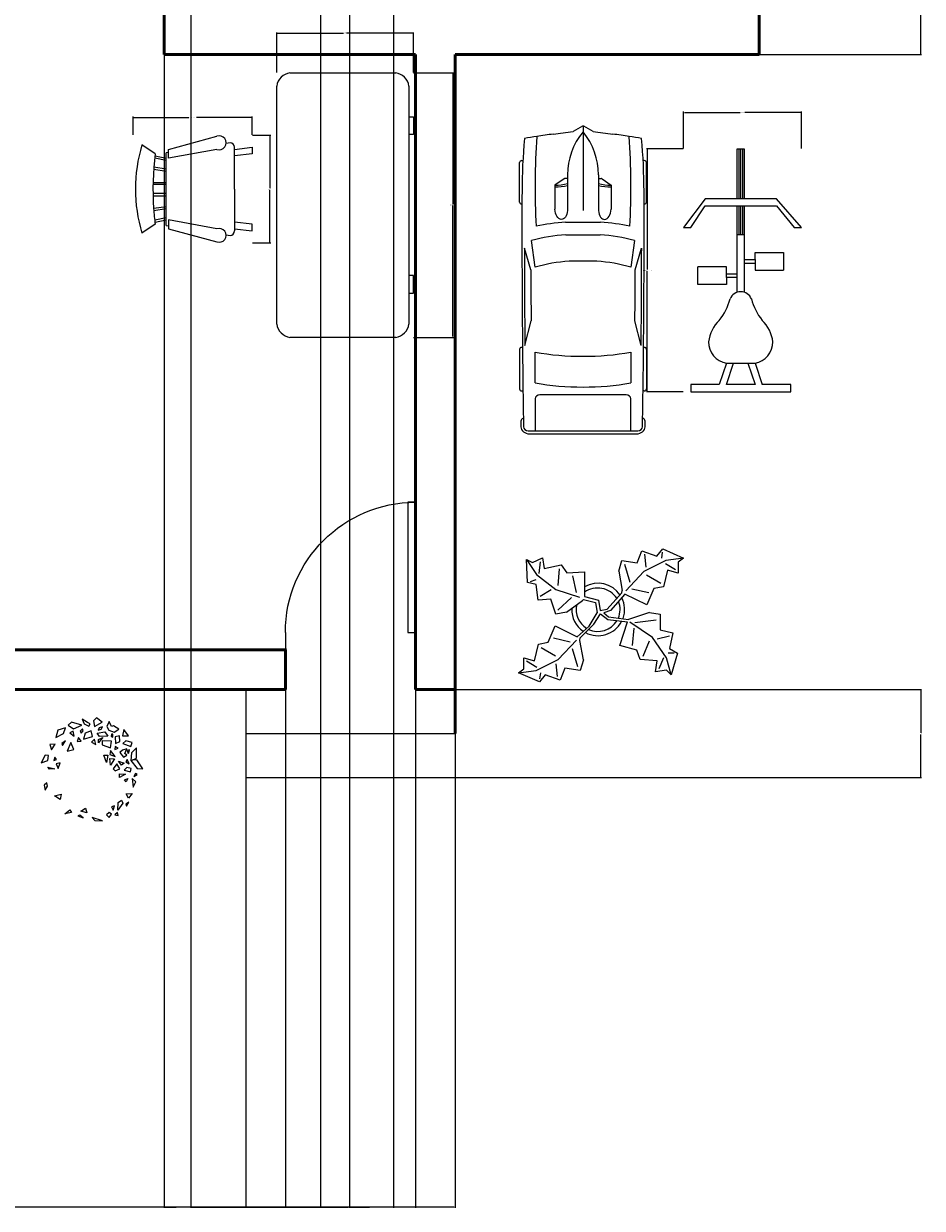
# Model space of a CAD drawing. Units: inches. Extents: x 177 to 602, y 30 to 608.
# Tile 2 of 4: x 398 to 602, y 30 to 299. Entities that reach past the tile are written whole.
import ezdxf

# ---------------------------------------------------------------- set-up
doc = ezdxf.new("R2010")
doc.units = ezdxf.units.IN
doc.header["$MEASUREMENT"] = 0
for name, color, linetype, lineweight in [('A-ANNO-DIMS', 2, 'Continuous', 18), ('A-DOOR', 3, 'Continuous', 25), ('A-EQPM', 9, 'Continuous', 18), ('A-FLOR-STRS', 7, 'Continuous', 25), ('A-FURN', 8, 'Continuous', 18), ('A-WALL', 7, 'Continuous', 50), ('C-PRKG-VEHL', 8, 'Continuous', 13), ('L-PLNT', 94, 'Continuous', 13)]:
    doc.layers.add(name, color=color, linetype=linetype, lineweight=lineweight)
doc.styles.get("Standard").update_dxf_attribs({"font": 'arial.ttf'})
doc.dimstyles.get("Standard").update_dxf_attribs({"dimtxt": 0.18, "dimasz": 0.18, "dimexe": 0.18, "dimexo": 0.0625, "dimgap": 0.09, "dimtad": 0, "dimtih": 1, "dimtoh": 1, "dimdec": 1, "dimzin": 0, "dimdsep": 46, "dimlunit": 4, "dimtxsty": 'Standard', "dimcen": 0.09, "dimadec": 0, "dimazin": 0, "dimtfac": 1, "dimtdec": 1, "dimtofl": 0, "dimtmove": 0, "dimatfit": 3, "dimfxl": 1, "dimtolj": 1, "dimtzin": 0, "dimarcsym": 0})

# ---------------------------------------------------------------- blocks, each defined once
blk = doc.blocks.new('*U3')
for p, q in [((-750, 0), (-750, 100)), ((0, 0), (0, 100))]:
    blk.add_line(p, q)
blk.add_lwpolyline([(0, 0), (0, -750), (-43.75, -750), (-43.75, 0)], close=True)
blk.add_arc((0, 0), 750, 180, 270)
blk = doc.blocks.new('*U9')
for points in [[(-4.43, 11.05), (-5.18, 10.36), (-3.96, 9.49), (-2.07, 10.36)], [(-2, 11.66), (-1.6, 10.62), (-0.52, 10.1), (-0.18, 10.62), (-0.79, 10.96)], [(1.24, 12), (0.56, 11.31), (0.76, 10.01), (2.52, 11.05)], [(4.14, 11.14), (3.6, 10.01), (4, 9.23), (5.22, 8.71), (6.3, 9.41), (5.08, 10.19), (4.61, 10.01)], [(-5.78, 9.75), (-7.54, 9.23), (-8.01, 7.5), (-6.26, 8.45)], [(-4.84, 8.63), (-3.83, 7.85), (-4.03, 8.97)], [(-1.94, 9.49), (-2.48, 8.97), (-2.27, 8.54), (-1.8, 9.06)], [(0.02, 9.06), (-1.33, 8.54), (-1.73, 7.16), (0.29, 7.76)], [(1.37, 8.54), (3.13, 8.8), (3.8, 7.85), (1.91, 7.76)], [(2.59, 9.93), (1.84, 9.75), (1.64, 9.23), (2.32, 9.41)], [(4.61, 8.28), (4.54, 7.76), (4.95, 7.59), (4.95, 8.28)], [(7.45, 9.32), (7.11, 7.94), (8.52, 7.94)], [(-8.14, 6.03), (-9.36, 5.95), (-9.02, 4.73)], [(-5.78, 6.81), (-6.66, 6.21), (-6.52, 5.69)], [(-4.57, 6.38), (-5.45, 4.47), (-3.89, 4.82)], [(-2.88, 7.5), (-3.15, 6.64), (-2.27, 6.72)], [(0.76, 7.16), (0.09, 6.46), (1.1, 5.95)], [(1.71, 6.29), (1.71, 7.07), (2.65, 7.5), (2.11, 6.9)], [(2.52, 6.81), (2.52, 5.86), (4.41, 5.17), (4.61, 6.72)], [(5.49, 5.51), (5.42, 4.82), (6.16, 5.08)], [(6.43, 7.94), (5.49, 7.68), (5.56, 6.21), (6.5, 6.64)], [(7.85, 6.81), (7.18, 6.21), (9, 5.51), (9.33, 6.38)], [(-11.32, 1.79), (-9.83, 2.31), (-9.63, 3.44), (-10.44, 3.52)], [(-8.21, 3.09), (-8.48, 2.31), (-7.87, 2.57)], [(3.53, 1.88), (2.86, 3.52), (3.8, 3.52)], [(4.41, 4.56), (4.27, 3.7), (5.49, 3.26)], [(4.27, 2.74), (5.29, 2.66), (4.41, 1.27)], [(8.12, 4.99), (7.11, 4.65), (6.5, 4.13), (7.38, 3.09), (8.12, 3.52), (7.65, 3.87)], [(8.73, 4.73), (8.19, 4.56), (8.39, 3.87), (8.59, 4.04)], [(10.28, 5.17), (9.2, 4.04), (9, 2.31), (10.48, 0.49), (11.76, 0.41), (10.35, 2.48), (9.33, 2.4), (10.28, 2.83)], [(-8.21, 0.41), (-9.43, 0.32), (-9.83, 0.84)], [(-7, 1.79), (-7.94, 1.53), (-7.47, 0.49)], [(5.83, 1.53), (5.02, 0.41), (5.49, -0.02), (6.5, 0.41)], [(7.51, 1.71), (6.91, 1.27), (6.23, 2.14)], [(8.12, 0.75), (7.51, 0.15), (8.93, -0.28), (9.13, 0.49)], [(8.19, 2.57), (7.92, 2.05), (8.66, 1.53)], [(7.78, -0.8), (6.43, -1.5), (6.43, -0.72)], [(8.32, -1.75), (7.98, -2.53), (7.58, -2.1)], [(9.33, -1.75), (9.54, -3.74), (10.14, -2.53)], [(10.08, -0.63), (9.74, -1.32), (10.48, -0.89)], [(-10.03, -2.71), (-10.64, -3.31), (-10.44, -4.44), (-9.9, -3.49)], [(-8.28, -5.73), (-6.79, -5.3), (-7, -6.51)], [(9.33, -5.13), (8.46, -6.25), (7.98, -5.22)], [(5.29, -7.98), (4.61, -8.16), (5.02, -8.94)], [(6.1, -8.94), (6.16, -7.21), (6.91, -6.69), (7.24, -7.38)], [(8.05, -8.07), (8.59, -7.12), (7.92, -7.55)], [(-4.84, -8.85), (-4.43, -9.45), (-5.99, -9.8)], [(-2.54, -10.06), (-3.02, -10.23), (-1.8, -10.67)], [(-2.34, -9.2), (-1.26, -8.5), (-0.99, -9.54)], [(0.22, -10.58), (0.83, -11.27), (2.59, -11.36)], [(4.07, -9.45), (3.53, -9.97), (4.07, -10.58), (4.61, -9.89)], [(6.03, -9.45), (5.42, -9.97), (6.16, -10.15)]]:
    blk.add_lwpolyline(points, close=True)
blk = doc.blocks.new('Chair - Rocking')
for p, q in [((-8, -4.5), (-10, -1.5)), ((8, -4.5), (10, -1.5)), ((-7.5, -4.5), (-7, -7)), ((-6.5, -7), (-7.02225, -4.43)), ((-4.5, -7), (-4.96674, -4.19951)), ((-4, -7), (-4.40532, -4.16272)), ((-1.5, -4.05012), (-1.5, -7)), ((-1, -7), (-1, -4.05012)), ((1, -7), (1, -4.04655)), ((1.5, -4.05012), (1.5, -7)), ((4, -7), (4.40187, -4.18694)), ((4.5, -7), (4.96761, -4.19437)), ((6.5, -7), (7, -4.4057)), ((7.5, -4.5), (7, -7)), ((-9, -7.5), (-12, -18.49999)), ((-7, -7.5), (-9, -7.5)), ((-9, -18.49999), (-7, -7.5)), ((-8.23428, -6.99939), (-8.3093, -7.47958)), ((-8.23041, -7), (8.23915, -7)), ((7, -7.5), (9, -7.5)), ((9, -18.49999), (7, -7.5)), ((8.31071, -7.48854), (8.23449, -7.00073)), ((9, -7.5), (12, -18.49999)), ((-10.36644, -20.64523), (-10.5, -21.49999)), ((10.5, -21.49999), (10.3575, -20.58798)), ((-9, -22.49999), (-9.5, -26.49999)), ((0, -22.49999), (-9.5, -22.49999)), ((-8, -26.49999), (-7.5, -22.49999)), ((0, -22.49999), (9.5, -22.49999)), ((8, -26.49999), (7.5, -22.49999)), ((9, -22.49999), (9.5, -26.49999)), ((-9.5, -26.49999), (-8, -26.49999)), ((9.5, -26.49999), (8, -26.49999))]:
    blk.add_line(p, q)
for centre, radius, start, end in [((0, -34.08333), 34.08333, 72.93847, 107.0615), ((0, -68.25004), 64.25, 93.92211, 97.15267), ((0, -68.25004), 64.25, 82.84733, 93.92211), ((-10.5, -18.99999), 1.58114, 161.5651, 18.43495), ((10.5, -18.99999), 1.58114, 161.5651, 18.43495), ((-9.5, -21.49999), 1, 180, 270), ((9.5, -21.49999), 1, 270, 0)]:
    blk.add_arc(centre, radius, start, end)
blk = doc.blocks.new('Desk - 30 x 60 in.')
for p, q in [((-26.999995, 0), (26.999995, 0)), ((-29.999995, -27), (-29.999995, -3)), ((29.999995, -3), (29.999995, -27)), ((26.999995, -30), (-26.999995, -30)), ((-20.000005, -30), (-20.000005, -31)), ((-20.000005, -31), (-16.000005, -31)), ((-16.000005, -31), (-16.000005, -30)), ((15.999995, -31), (15.999995, -30)), ((19.999995, -31), (15.999995, -31)), ((19.999995, -30), (19.999995, -31))]:
    blk.add_line(p, q)
for centre, start, end in [((-26.499995, -3.5), 98.1301, 171.8699), ((26.499995, -3.5), 8.130102, 81.8699), ((-26.499995, -26.5), 188.1301, 261.8699), ((26.499995, -26.5), 278.1301, 351.8699)]:
    blk.add_arc(centre, 3.535534, start, end)
blk = doc.blocks.new('Plant - Rubber or Philodendron')
for p, q in [((8.8871, 10.7908), (9.9809, 13.4933)), ((9.9809, 13.4933), (13.3837, 12.301)), ((13.3837, 12.301), (14.68, 13.9039)), ((14.68, 13.9039), (19.3848, 11.8146)), ((-16.2005, 11.4774), (-13.9899, 8.1064)), ((-16.2005, 11.4774), (-14.8639, 10.7964)), ((-16.0159, 6.3329), (-16.2005, 11.4774)), ((-14.8639, 10.7964), (-12.6195, 11.8975)), ((-13.3174, 8.325), (-13.0735, 11.0065)), ((-12.6195, 11.8975), (-12.1909, 9.4345)), ((4.6914, 8.8812), (5.3859, 11.2828)), ((5.3859, 11.2828), (8.8871, 10.7908)), ((15.3859, 11.3055), (10.3916, 8.7942)), ((10.5828, 12.6946), (10.8893, 9.7953)), ((14.5816, 13.2037), (14.3848, 11.8033)), ((19.3848, 11.8146), (15.3859, 11.3055)), ((19.3848, 11.8146), (18.1868, 10.9119)), ((18.1868, 10.9119), (18.1925, 8.4119)), ((-13.9899, 8.1064), (-9.5434, 4.7185)), ((-12.1909, 9.4345), (-8.3829, 10.3)), ((-8.8369, 9.409), (-9.0894, 5.6095)), ((-8.3829, 10.3), (-7.0549, 8.501)), ((-7.0549, 8.501), (-3.0284, 8.6941)), ((-3.0284, 8.6941), (-3.0709, 3.1041)), ((4.6914, 8.8812), (5.5014, 4.4831)), ((5.9878, 10.4842), (7.1971, 6.3869)), ((10.3916, 8.7942), (6.2847, 4.4028)), ((15.7909, 9.1065), (14.8995, 5.3044)), ((15.2875, 10.6053), (17.5907, 9.2105)), ((18.1925, 8.4119), (15.7909, 9.1065)), ((-14.0069, 5.8704), (-16.0159, 6.3329)), ((-15.3434, 6.5514), (-13.9984, 6.9884)), ((-13.5868, 2.2894), (-14.0069, 5.8704)), ((-4.8529, 4.012), (-5.7184, 7.82)), ((14.2977, 6.1031), (10.9934, 7.9956)), ((-13.1329, 3.1804), (-10.6614, 4.727)), ((-9.5434, 4.7185), (-4.1917, 2.9888)), ((-9.1318, 0.0195), (-5.9793, 2.9025)), ((-3.0709, 3.1041), (0.0797, 2.3163)), ((2.1141, 0.2298), (5.4346, 3.9146)), ((6.1032, 3.6844), (2.8262, -0.031)), ((5.4346, 3.9146), (5.5014, 4.4831)), ((11.1089, 1.1958), (6.1032, 3.6844)), ((7.7005, 4.8881), (11.5025, 3.9967)), ((12.7005, 4.8994), (11.1089, 1.1958)), ((14.8995, 5.3044), (12.7005, 4.8994)), ((-10.6784, 2.491), (-13.5868, 2.2894)), ((-9.5858, -0.8715), (-10.6784, 2.491)), ((-7.1228, -0.443), (-3.5248, 2.2131)), ((-3.5248, 2.2131), (-3.3011, 2.4355)), ((-3.3011, 2.4355), (-0.5306, 1.7947)), ((-0.5306, 1.7947), (-0.2255, -0.5527)), ((-0.5306, 1.7947), (-0.5306, 1.7947)), ((0.0797, 2.3163), (0.4866, -0.031)), ((0.4866, -0.031), (2.1141, 0.2298)), ((-7.1228, -0.443), (-9.5858, -0.8715)), ((-2.019, -3.6148), (-0.2255, -0.5527)), ((-0.9375, -3.1608), (0.5883, -0.8135)), ((0.5883, -0.8135), (2.2447, -2.0916)), ((2.8262, -0.031), (1.3003, -0.5527)), ((1.3003, -0.5527), (2.4193, -1.4655)), ((2.2447, -2.0916), (6.7108, -2.6626)), ((2.4193, -1.4655), (6.895, -2.1175)), ((4.943, -7.9659), (6.7108, -2.6626)), ((11.6605, -0.5413), (6.895, -2.1175)), ((12.3677, -6.1981), (7.219, -2.6772)), ((8.3544, -2.7453), (13.1973, -2.1704)), ((11.6605, -0.5413), (14.1354, -0.8948)), ((14.1354, -0.8948), (14.1354, -4.4304)), ((-11.3237, -7.2629), (-9.7321, -3.5593)), ((-9.7321, -3.5593), (-4.7264, -6.0479)), ((-2.019, -3.6148), (-4.7264, -6.0479)), ((-4.0579, -6.2781), (-0.9375, -3.1608)), ((8.125, -4.0768), (7.7715, -7.9659)), ((14.1354, -4.4304), (16.9638, -5.1375)), ((16.9638, -5.1375), (16.2567, -8.673)), ((-14.4141, -11.4699), (-13.5228, -7.6679)), ((-13.5228, -7.6679), (-11.3237, -7.2629)), ((-6.3237, -7.2516), (-10.1257, -6.3602)), ((-9.0148, -11.1577), (-4.9047, -6.8122)), ((-4.1246, -6.8466), (-4.0579, -6.2781)), ((-3.3146, -11.2447), (-4.1246, -6.8466)), ((8.8321, -9.0266), (4.943, -7.9659)), ((10.2463, -10.4408), (11.6605, -6.9053)), ((15.5496, -10.7943), (12.3677, -6.1981)), ((16.2567, -5.8446), (13.4283, -6.5517)), ((-12.921, -8.4665), (-9.6166, -10.359)), ((-4.611, -12.8477), (-5.8203, -8.7504)), ((9.5392, -11.1479), (8.8321, -9.0266)), ((17.3174, -9.7337), (15.9032, -9.7337)), ((16.2567, -8.673), (18.0245, -9.7337)), ((18.0245, -9.7337), (16.6103, -14.6834)), ((-18.008, -14.1781), (-16.8101, -13.2754)), ((-16.8157, -10.7754), (-14.4141, -11.4699)), ((-16.8101, -13.2754), (-16.8157, -10.7754)), ((-13.9107, -12.9688), (-16.2139, -11.574)), ((-14.0091, -13.669), (-9.0148, -11.1577)), ((-9.206, -15.0581), (-9.5126, -12.1588)), ((-7.5103, -13.1543), (-8.6042, -15.8568)), ((-4.0092, -13.6463), (-7.5103, -13.1543)), ((-3.3146, -11.2447), (-4.0092, -13.6463)), ((13.4283, -11.5015), (9.5392, -11.1479)), ((13.0748, -13.9763), (13.4283, -11.5015)), ((14.8425, -10.7943), (13.7819, -13.2692)), ((16.6103, -14.6834), (15.5496, -10.7943)), ((-18.008, -14.1781), (-14.0091, -13.669)), ((-13.3032, -16.2674), (-18.008, -14.1781)), ((-12.0069, -14.6645), (-13.3032, -16.2674)), ((-13.2048, -15.5672), (-13.008, -14.1668)), ((-8.6042, -15.8568), (-12.0069, -14.6645)), ((15.5496, -13.6228), (13.0748, -13.9763)), ((16.6103, -14.6834), (15.5496, -13.6228))]:
    blk.add_line(p, q)
for centre, radius, start, end in [((0, 0), 6.1275, 34.37569, 120.1028), ((-0.0601, -0.2075), 5.2461, 33.82192, 124.9414), ((-0.098, 0.1364), 6.1288, 341.2017, 26.09184), ((0.0308, 0.1664), 6, 178.6147, 235.1169), ((0.0308, 0.1664), 5, 168.1647, 238.6725), ((-0.2664, 0.1682), 5.2775, 338.4094, 20.03007), ((-0.0234, 0.3825), 6.1492, 242.5812, 331.2714), ((-0.1102, 0.4886), 5.2883, 247.3711, 327.472)]:
    blk.add_arc(centre, radius, start, end)
blk = doc.blocks.new('*U31')
for p, q in [((21.1, 37.41), (21.1, 36.83)), ((46.55, 38.89), (22.35, 38.89)), ((47.8, 37.39), (47.8, 37.41)), ((135.45, 37.07), (135.45, 37.41)), ((136.7, 38.89), (160.9, 38.89)), ((162.15, 37.41), (162.15, 36.77)), ((70.03, 31.54), (86.41, 29.35)), ((87.99, 31.87), (74.76, 35.92)), ((134.31, 35.6), (119.29, 31.78)), ((138.42, 29.35), (157.25, 29.35)), ((186.47, 29.35), (167.01, 29.35)), ((186.47, -33.5), (186.47, 33.5)), ((188.4, -32.76), (188.4, 32.76)), ((164.52, 26.39), (164.52, -26.39)), ((32.27, 11.63), (36.13, 17.17)), ((36.13, 17.17), (50.94, 17.17)), ((29.77, 9.51), (51.68, 9.51)), ((32.12, 9.51), (32.12, 11.15)), ((58.92, -10.77), (58.92, 10.77)), ((66.55, -10.53), (66.55, 10.53)), ((82.74, 8.5), (82.74, -8.5)), ((186.47, -10.53), (186.47, 10.53)), ((3.27, 6.13), (0.1, 0.41)), ((0, 0), (51.68, 0)), ((0.1, -0.41), (3.27, -6.13)), ((29.77, -9.51), (51.68, -9.51)), ((32.12, -9.51), (32.12, -11.15)), ((32.27, -11.63), (36.13, -17.17)), ((36.13, -17.17), (50.94, -17.17)), ((86.41, -29.35), (70.03, -31.54)), ((87.99, -31.87), (74.76, -35.92)), ((134.31, -35.6), (119.29, -31.78)), ((157.25, -29.35), (138.42, -29.35)), ((167.01, -29.35), (186.47, -29.35)), ((21.1, -37.41), (21.1, -36.83)), ((46.55, -38.89), (22.35, -38.89)), ((47.8, -37.39), (47.8, -37.41)), ((135.45, -37.07), (135.45, -37.41)), ((136.7, -38.89), (160.9, -38.89)), ((162.15, -37.41), (162.15, -36.77))]:
    blk.add_line(p, q)
for centre, major_axis, ratio, start_param, end_param in [((41.19, -490.86), (0, 528.23), 0.842304, 0.00281, 0.075598), ((22.35, 37.41), (0, -1.48), 0.842304, 3.141593, 4.712389), ((64.48, -10555.62), (0, 10593.03), 0.842304, -0.013397, 0.002797), ((46.55, 37.41), (0, 1.48), 0.842304, -1.570796, 0), ((136.7, 37.41), (0, -1.48), 0.842304, 3.141593, 4.712389), ((160.9, 37.41), (0, 1.48), 0.842304, -1.570796, 0), ((180.63, 35.84), (0, 2.22), 0.842304, -0.013017, 1.249894), ((64.48, -10556.36), (0, 10595.31), 0.842304, -0.013397, -0.013017), ((183.98, 33.5), (0, -2.96), 0.842304, 1.570796, 3.128196), ((183.98, 32.76), (0, -5.25), 0.842304, 1.570796, 3.128196), ((266.03, -27.52), (0, 313.31), 0.842304, 1.367076, 1.39176), ((37.47, -593.96), (0, -623.33), 0.842304, 3.096046, 3.200911), ((135.29, 5.39), (0, 81.77), 0.842304, 1.245306, 1.50788), ((64.48, -10555.62), (0, -10591.55), 0.842304, 3.133765, 3.140441), ((149.6, 2.8), (0, -79.58), 0.842304, 4.372215, 4.640744), ((95.79, -3666.35), (0, -3698.24), 0.842304, 3.134049, 3.144098), ((17.08, 0), (0, 147.02), 0.842304, 4.511394, 4.913384), ((35.91, 0), (0, 147.02), 0.842304, 4.511394, 4.913384), ((167.01, 26.39), (0, 2.96), 0.842304, 0, 1.570796), ((259.18, -27.52), (0, -305.3), 0.842304, 4.528606, 4.561838), ((134.4, 5.39), (0, -89.78), 0.842304, 4.449482, 4.652344), ((-204.49, 52.4), (0, -250.96), 0.842304, 1.385369, 1.434372), ((13.04, 17.01), (0, 27.42), 0.842304, 4.435146, 4.718221), ((14.2, 17.01), (0, 27.42), 0.842304, 4.435146, 4.718221), ((50.79, 13.34), (6.34, -0.36), 0.603834, -1.395552, 1.581315), ((29.77, -46.66), (0, 56.17), 0.842304, 0, 0.590319), ((32.75, 11.15), (0, 0.74), 0.842304, 0.879714, 1.570796), ((0.62, 0), (0, -0.74), 0.842304, 4.131459, 5.293319), ((-204.49, -52.4), (0, 250.96), 0.842304, -1.434372, -1.385369), ((29.77, 46.66), (0, 56.17), 0.842304, 2.551274, 3.141593), ((32.75, -11.15), (0, -0.74), 0.842304, 4.712389, 5.403472), ((13.04, -17.01), (0, -27.42), 0.842304, 1.564964, 1.848039), ((14.2, -17.01), (0, -27.42), 0.842304, 1.564964, 1.848039), ((134.4, -5.39), (0, -89.78), 0.842304, -1.510751, -1.307889), ((135.29, -5.39), (0, -81.77), 0.842304, -1.50788, -1.245306), ((149.6, -2.8), (0, -79.58), 0.842304, -1.499151, -1.230623), ((259.18, 27.52), (0, 305.3), 0.842304, 1.721348, 1.754579), ((266.03, 27.52), (0, 313.31), 0.842304, 1.749832, 1.774517), ((37.47, 593.96), (0, -623.33), 0.842304, -0.059319, 0.045547), ((167.01, -26.39), (0, -2.96), 0.842304, 4.712389, 6.283185), ((41.19, 490.86), (0, -528.23), 0.842304, -0.075598, -0.00281), ((64.48, 10555.62), (0, -10591.55), 0.842304, 0.001152, 0.007828), ((95.79, 3666.35), (0, -3698.24), 0.842304, -0.002505, 0.007544), ((183.98, -33.5), (0, 2.96), 0.842304, 3.15499, 4.712389), ((183.98, -32.76), (0, -5.25), 0.842304, 0.013397, 1.570796), ((22.35, -37.41), (0, 1.48), 0.842304, 1.570796, 3.141593), ((64.48, 10555.62), (0, 10593.03), 0.842304, 3.138796, 3.15499), ((46.55, -37.41), (0, -1.48), 0.842304, 0, 1.570796), ((136.7, -37.41), (0, -1.48), 0.842304, -1.570796, 0), ((160.9, -37.41), (0, 1.48), 0.842304, 3.141593, 4.712389), ((180.63, -35.84), (0, -2.22), 0.842304, -1.249894, 0.013017), ((64.48, 10556.36), (0, 10595.31), 0.842304, 3.15461, 3.15499)]:
    blk.add_ellipse(centre, major_axis=major_axis, ratio=ratio, start_param=start_param, end_param=end_param)
at = {"extrusion": (0, 0, -1)}
blk.add_ellipse((50.79, -13.34), major_axis=(6.34, 0.36), ratio=0.603834, start_param=-1.395552, end_param=1.581315, dxfattribs=at)
blk = doc.blocks.new('Exercise Bike')
for p, q in [((-0.75, 10), (-0.75, 17)), ((-0.75, 17), (0.25, 17)), ((-0.5, 17), (-0.5, 9.9929)), ((-0.25, 10), (-0.25, 17)), ((0, 17), (0, 9.9929)), ((0.25, 17), (0.25, 10)), ((-5.25, 10), (-8.25, 6)), ((-0.75, 10), (-5.25, 10)), ((4.75, 10), (-0.75, 10)), ((8.25, 6), (4.75, 10)), ((-7.25, 6), (-5.25, 9)), ((-5.25, 9), (4.75, 9)), ((-0.75, 5), (-0.75, 9)), ((-0.5, 8.9396), (-0.5, 5)), ((-0.25, 5), (-0.25, 9)), ((0, 8.9396), (0, 5)), ((0.25, 9), (0.25, 5)), ((4.75, 9), (7.25, 6)), ((-8.25, 6), (-7.25, 6)), ((-0.75, -3.0635), (-0.75, 5)), ((-0.75, 5), (0.25, 5)), ((0.25, 5), (0.25, -3.0635)), ((7.25, 6), (8.25, 6)), ((1.75, 2.5), (5.75, 2.5)), ((1.75, 1.5), (1.75, 2.5)), ((5.75, 2.5), (5.75, 0)), ((-6.25, -2), (-6.25, 0.5)), ((-2.25, 0.5), (-6.25, 0.5)), ((-2.25, -0.5), (-2.25, 0.5)), ((0.25, 1.5), (1.75, 1.5)), ((0.25, 1), (1.75, 1)), ((1.75, 1.5), (1.75, 0)), ((1.75, 0), (5.75, 0)), ((-2.25, -0.5), (-0.75, -0.5)), ((-2.25, -1), (-2.25, -0.5)), ((-2.25, -1), (-2.25, -2)), ((-0.75, -1), (-2.25, -1)), ((-2.25, -2), (-6.25, -2)), ((-2.25, -13), (-3.25, -16)), ((-2.25, -16), (-1.25, -13)), ((-2.25, -13), (1.75, -13)), ((0.75, -13), (1.75, -16)), ((1.75, -13), (2.75, -16)), ((-7.25, -16), (-7.25, -17)), ((-4.75, -16), (-7.25, -16)), ((-3.25, -16), (-4.75, -16)), ((1.75, -16), (-2.25, -16)), ((6.75, -16), (2.75, -16)), ((6.75, -17), (6.75, -16)), ((-7.25, -17), (6.75, -17))]:
    blk.add_line(p, q)
for centre, radius, start, end in [((-0.25, -4.625), 1.625, 22.61987, 157.3801), ((-9.6692, -1.9154), 8.1889, 321.6175, 345.2525), ((9.1691, -1.9154), 8.1889, 194.7476, 218.3825), ((0.1685, -10.5843), 4.9531, 133.6443, 173.2256), ((-0.6686, -10.5843), 4.9531, 6.774486, 46.35562), ((-1.7006, -10.0005), 3.0494, 179.9906, 259.6205), ((1.2006, -10.0005), 3.0494, 280.3795, 0.009389)]:
    blk.add_arc(centre, radius, start, end)
blk = doc.blocks.new('*D65')
at = {"layer": 'A-ANNO-DIMS', "color": 0, "lineweight": -2, "transparency": 16777216}
for p, q in [((423.27, 273.93), (423.27, 278.1)), ((423.45, 277.92), (435.87, 277.92)), ((450.09, 277.92), (437.67, 277.92)), ((450.27, 273.93), (450.27, 278.1))]:
    blk.add_line(p, q, dxfattribs=at)
at = {"layer": 'A-ANNO-DIMS', "color": 0, "transparency": 16777216}
for points in [[(423.45, 277.95), (423.45, 277.89), (423.27, 277.92)], [(450.09, 277.95), (450.09, 277.89), (450.27, 277.92)]]:
    blk.add_solid(points, dxfattribs=at)
at = {"layer": 'Defpoints', "color": 0, "transparency": 16777216}
for p in [(423.27, 277.92), (423.27, 273.87), (450.27, 273.87)]:
    blk.add_point(p, dxfattribs=at)
at = {"layer": 'A-ANNO-DIMS', "color": 0, "transparency": 16777216, "insert": (436.77, 277.92), "char_height": 0.18, "attachment_point": 5}
blk.add_mtext('\\A1;ROCKER 2\'-3"', dxfattribs=at)
blk = doc.blocks.new('*D66')
at = {"layer": 'A-ANNO-DIMS', "color": 0, "lineweight": -2, "transparency": 16777216}
for p, q in [((450.33, 273.87), (454.5, 273.87)), ((454.32, 273.69), (454.32, 261.84)), ((454.32, 249.62), (454.32, 261.47)), ((450.33, 249.44), (454.5, 249.44))]:
    blk.add_line(p, q, dxfattribs=at)
at = {"layer": 'A-ANNO-DIMS', "color": 0, "transparency": 16777216}
for points in [[(454.29, 273.69), (454.35, 273.69), (454.32, 273.87)], [(454.29, 249.62), (454.35, 249.62), (454.32, 249.44)]]:
    blk.add_solid(points, dxfattribs=at)
at = {"layer": 'Defpoints', "color": 0, "transparency": 16777216}
for p in [(450.27, 273.87), (454.32, 273.87), (450.27, 249.44)]:
    blk.add_point(p, dxfattribs=at)
at = {"layer": 'A-ANNO-DIMS', "color": 0, "transparency": 16777216, "insert": (454.32, 261.65), "char_height": 0.18, "attachment_point": 5}
blk.add_mtext('\\A1;2\'-0 1/2"', dxfattribs=at)
blk = doc.blocks.new('*D67')
at = {"layer": 'A-ANNO-DIMS', "color": 0, "lineweight": -2, "transparency": 16777216}
for p, q in [((486.92, 288.01), (496.04, 288.01)), ((495.86, 287.83), (495.86, 258.19)), ((495.86, 228.19), (495.86, 257.82)), ((486.92, 228.01), (496.04, 228.01))]:
    blk.add_line(p, q, dxfattribs=at)
at = {"layer": 'A-ANNO-DIMS', "color": 0, "transparency": 16777216}
for points in [[(495.83, 287.83), (495.89, 287.83), (495.86, 288.01)], [(495.83, 228.19), (495.89, 228.19), (495.86, 228.01)]]:
    blk.add_solid(points, dxfattribs=at)
at = {"layer": 'Defpoints', "color": 0, "transparency": 16777216}
for p in [(486.86, 288.01), (495.86, 288.01), (486.86, 228.01)]:
    blk.add_point(p, dxfattribs=at)
at = {"layer": 'A-ANNO-DIMS', "color": 0, "transparency": 16777216, "insert": (495.86, 258.01), "char_height": 0.18, "attachment_point": 5}
blk.add_mtext('\\A1;DESK 5\'-0"', dxfattribs=at)
blk = doc.blocks.new('*D68')
at = {"layer": 'A-ANNO-DIMS', "color": 0, "lineweight": -2, "transparency": 16777216}
for p, q in [((455.86, 288.07), (455.86, 297.19)), ((456.04, 297.01), (471.03, 297.01)), ((486.68, 297.01), (471.69, 297.01)), ((486.86, 288.07), (486.86, 297.19))]:
    blk.add_line(p, q, dxfattribs=at)
at = {"layer": 'A-ANNO-DIMS', "color": 0, "transparency": 16777216}
for points in [[(456.04, 297.04), (456.04, 296.98), (455.86, 297.01)], [(486.68, 297.04), (486.68, 296.98), (486.86, 297.01)]]:
    blk.add_solid(points, dxfattribs=at)
at = {"layer": 'Defpoints', "color": 0, "transparency": 16777216}
for p in [(455.86, 297.01), (455.86, 288.01), (486.86, 288.01)]:
    blk.add_point(p, dxfattribs=at)
at = {"layer": 'A-ANNO-DIMS', "color": 0, "transparency": 16777216, "insert": (471.36, 297.01), "char_height": 0.18, "attachment_point": 5}
blk.add_mtext('\\A1;2\'-7"', dxfattribs=at)
blk = doc.blocks.new('*D71')
at = {"layer": 'A-ANNO-DIMS', "color": 0, "lineweight": -2, "transparency": 16777216}
for p, q in [((548.13, 270.77), (539.75, 270.77)), ((539.93, 270.59), (539.93, 243.4)), ((539.93, 215.84), (539.93, 243.03)), ((548.13, 215.66), (539.75, 215.66))]:
    blk.add_line(p, q, dxfattribs=at)
at = {"layer": 'A-ANNO-DIMS', "color": 0, "transparency": 16777216}
for points in [[(539.9, 270.59), (539.96, 270.59), (539.93, 270.77)], [(539.9, 215.84), (539.96, 215.84), (539.93, 215.66)]]:
    blk.add_solid(points, dxfattribs=at)
at = {"layer": 'Defpoints', "color": 0, "transparency": 16777216}
for p in [(539.93, 270.77), (548.19, 270.77), (548.19, 215.66)]:
    blk.add_point(p, dxfattribs=at)
at = {"layer": 'A-ANNO-DIMS', "color": 0, "transparency": 16777216, "insert": (539.93, 243.22), "char_height": 0.18, "attachment_point": 5}
blk.add_mtext('\\A1;EXERCISE BIKE 4\'-7"', dxfattribs=at)
blk = doc.blocks.new('*D72')
at = {"layer": 'A-ANNO-DIMS', "color": 0, "lineweight": -2, "transparency": 16777216}
for p, q in [((548.19, 270.83), (548.19, 279.22)), ((548.37, 279.04), (561.03, 279.04)), ((574.76, 279.04), (562.11, 279.04)), ((574.94, 270.83), (574.94, 279.22))]:
    blk.add_line(p, q, dxfattribs=at)
at = {"layer": 'A-ANNO-DIMS', "color": 0, "transparency": 16777216}
for points in [[(548.37, 279.07), (548.37, 279.01), (548.19, 279.04)], [(574.76, 279.07), (574.76, 279.01), (574.94, 279.04)]]:
    blk.add_solid(points, dxfattribs=at)
at = {"layer": 'Defpoints', "color": 0, "transparency": 16777216}
for p in [(574.94, 279.04), (548.19, 270.77), (574.94, 270.77)]:
    blk.add_point(p, dxfattribs=at)
at = {"layer": 'A-ANNO-DIMS', "color": 0, "transparency": 16777216, "insert": (561.57, 279.04), "char_height": 0.18, "attachment_point": 5}
blk.add_mtext('\\A1;2\'-2 1/2"', dxfattribs=at)
blk = doc.blocks.new('*D73')
at = {"layer": 'A-ANNO-DIMS', "color": 0, "lineweight": -2, "transparency": 16777216}
for p, q in [((253.34, 148.07), (253.34, 30.54)), ((496.34, 128.07), (496.34, 30.54)), ((253.52, 30.72), (374.44, 30.72)), ((496.16, 30.72), (375.24, 30.72))]:
    blk.add_line(p, q, dxfattribs=at)
at = {"layer": 'A-ANNO-DIMS', "color": 0, "transparency": 16777216}
for points in [[(253.52, 30.75), (253.52, 30.69), (253.34, 30.72)], [(496.16, 30.75), (496.16, 30.69), (496.34, 30.72)]]:
    blk.add_solid(points, dxfattribs=at)
at = {"layer": 'Defpoints', "color": 0, "transparency": 16777216}
for p in [(253.34, 148.14), (496.34, 128.14), (496.34, 30.72)]:
    blk.add_point(p, dxfattribs=at)
at = {"layer": 'A-ANNO-DIMS', "color": 0, "transparency": 16777216, "insert": (374.84, 30.72), "char_height": 0.18, "attachment_point": 5}
blk.add_mtext('\\A1;20\'-3"', dxfattribs=at)
blk = doc.blocks.new('*D74')
at = {"layer": 'A-ANNO-DIMS', "color": 0, "lineweight": -2, "transparency": 16777216}
for p, q in [((565.4, 556.14), (602.22, 556.14)), ((602.04, 555.96), (602.04, 424.32)), ((602.04, 292.32), (602.04, 423.96)), ((565.4, 292.14), (602.22, 292.14))]:
    blk.add_line(p, q, dxfattribs=at)
at = {"layer": 'A-ANNO-DIMS', "color": 0, "transparency": 16777216}
for points in [[(602.01, 555.96), (602.07, 555.96), (602.04, 556.14)], [(602.01, 292.32), (602.07, 292.32), (602.04, 292.14)]]:
    blk.add_solid(points, dxfattribs=at)
at = {"layer": 'Defpoints', "color": 0, "transparency": 16777216}
for p in [(565.34, 556.14), (602.04, 556.14), (565.34, 292.14)]:
    blk.add_point(p, dxfattribs=at)
at = {"layer": 'A-ANNO-DIMS', "color": 0, "transparency": 16777216, "insert": (602.04, 424.14), "char_height": 0.18, "attachment_point": 5}
blk.add_mtext('\\A1;22\'-0"', dxfattribs=at)
blk = doc.blocks.new('*D77')
at = {"layer": 'A-ANNO-DIMS', "color": 0, "lineweight": -2, "transparency": 16777216}
for p, q in [((457.81, 148.07), (457.81, 30.54)), ((487.34, 148.07), (487.34, 30.54)), ((457.99, 30.72), (472.04, 30.72)), ((487.16, 30.72), (473.12, 30.72))]:
    blk.add_line(p, q, dxfattribs=at)
at = {"layer": 'A-ANNO-DIMS', "color": 0, "transparency": 16777216}
for points in [[(457.99, 30.75), (457.99, 30.69), (457.81, 30.72)], [(487.16, 30.75), (487.16, 30.69), (487.34, 30.72)]]:
    blk.add_solid(points, dxfattribs=at)
at = {"layer": 'Defpoints', "color": 0, "transparency": 16777216}
for p in [(457.81, 148.14), (487.34, 148.14), (487.34, 30.72)]:
    blk.add_point(p, dxfattribs=at)
at = {"layer": 'A-ANNO-DIMS', "color": 0, "transparency": 16777216, "insert": (472.58, 30.72), "char_height": 0.18, "attachment_point": 5}
blk.add_mtext('\\A1;2\'-5 1/2"', dxfattribs=at)
blk = doc.blocks.new('*D78')
at = {"layer": 'A-ANNO-DIMS', "color": 0, "lineweight": -2, "transparency": 16777216}
for p, q in [((448.81, 128.07), (448.81, 30.54)), ((496.34, 128.07), (496.34, 30.54)), ((448.99, 30.72), (471.97, 30.72)), ((496.16, 30.72), (473.18, 30.72))]:
    blk.add_line(p, q, dxfattribs=at)
at = {"layer": 'A-ANNO-DIMS', "color": 0, "transparency": 16777216}
for points in [[(448.99, 30.75), (448.99, 30.69), (448.81, 30.72)], [(496.16, 30.75), (496.16, 30.69), (496.34, 30.72)]]:
    blk.add_solid(points, dxfattribs=at)
at = {"layer": 'Defpoints', "color": 0, "transparency": 16777216}
for p in [(448.81, 128.14), (496.34, 128.14), (496.34, 30.72)]:
    blk.add_point(p, dxfattribs=at)
at = {"layer": 'A-ANNO-DIMS', "color": 0, "transparency": 16777216, "insert": (472.58, 30.72), "char_height": 0.18, "attachment_point": 5}
blk.add_mtext('\\A1;3\'-11 1/2"', dxfattribs=at)
blk = doc.blocks.new('*D84')
at = {"layer": 'A-ANNO-DIMS', "color": 0, "lineweight": -2, "transparency": 16777216}
for p, q in [((436.34, 379.07), (436.34, 30.54)), ((430.34, 374.22), (430.34, 30.54)), ((430.52, 30.72), (433.01, 30.72)), ((436.16, 30.72), (433.67, 30.72))]:
    blk.add_line(p, q, dxfattribs=at)
at = {"layer": 'A-ANNO-DIMS', "color": 0, "transparency": 16777216}
for points in [[(430.52, 30.75), (430.52, 30.69), (430.34, 30.72)], [(436.16, 30.75), (436.16, 30.69), (436.34, 30.72)]]:
    blk.add_solid(points, dxfattribs=at)
at = {"layer": 'Defpoints', "color": 0, "transparency": 16777216}
for p in [(436.34, 379.14), (430.34, 374.28), (430.34, 30.72)]:
    blk.add_point(p, dxfattribs=at)
at = {"layer": 'A-ANNO-DIMS', "color": 0, "transparency": 16777216, "insert": (433.34, 30.72), "char_height": 0.18, "attachment_point": 5}
blk.add_mtext('\\A1;0\'-6"', dxfattribs=at)
blk = doc.blocks.new('*D87')
at = {"layer": 'A-ANNO-DIMS', "color": 0, "lineweight": -2, "transparency": 16777216}
for p, q in [((436.34, 379.07), (436.34, 30.54)), ((465.79, 379.07), (465.79, 30.54)), ((436.52, 30.72), (450.53, 30.72)), ((465.61, 30.72), (451.61, 30.72))]:
    blk.add_line(p, q, dxfattribs=at)
at = {"layer": 'A-ANNO-DIMS', "color": 0, "transparency": 16777216}
for points in [[(436.52, 30.75), (436.52, 30.69), (436.34, 30.72)], [(465.61, 30.75), (465.61, 30.69), (465.79, 30.72)]]:
    blk.add_solid(points, dxfattribs=at)
at = {"layer": 'Defpoints', "color": 0, "transparency": 16777216}
for p in [(436.34, 379.14), (465.79, 379.14), (465.79, 30.72)]:
    blk.add_point(p, dxfattribs=at)
at = {"layer": 'A-ANNO-DIMS', "color": 0, "transparency": 16777216, "insert": (451.07, 30.72), "char_height": 0.18, "attachment_point": 5}
blk.add_mtext('\\A1;2\'-5 1/2"', dxfattribs=at)
blk = doc.blocks.new('*D92')
at = {"layer": 'A-ANNO-DIMS', "color": 0, "lineweight": -2, "transparency": 16777216}
for p, q in [((472.34, 373.07), (472.34, 30.54)), ((482.34, 373.07), (482.34, 30.54)), ((472.52, 30.72), (476.94, 30.72)), ((482.16, 30.72), (477.74, 30.72))]:
    blk.add_line(p, q, dxfattribs=at)
at = {"layer": 'A-ANNO-DIMS', "color": 0, "transparency": 16777216}
for points in [[(472.52, 30.75), (472.52, 30.69), (472.34, 30.72)], [(482.16, 30.75), (482.16, 30.69), (482.34, 30.72)]]:
    blk.add_solid(points, dxfattribs=at)
at = {"layer": 'Defpoints', "color": 0, "transparency": 16777216}
for p in [(472.34, 373.14), (482.34, 373.14), (482.34, 30.72)]:
    blk.add_point(p, dxfattribs=at)
at = {"layer": 'A-ANNO-DIMS', "color": 0, "transparency": 16777216, "insert": (477.34, 30.72), "char_height": 0.18, "attachment_point": 5}
blk.add_mtext('\\A1;0\'-10"', dxfattribs=at)
blk = doc.blocks.new('*D93')
at = {"layer": 'A-ANNO-DIMS', "color": 0, "lineweight": -2, "transparency": 16777216}
for p, q in [((496.4, 148.14), (602.22, 148.14)), ((602.04, 147.96), (602.04, 138.32)), ((602.04, 128.32), (602.04, 137.96)), ((496.4, 128.14), (602.22, 128.14))]:
    blk.add_line(p, q, dxfattribs=at)
at = {"layer": 'A-ANNO-DIMS', "color": 0, "transparency": 16777216}
for points in [[(602.01, 147.96), (602.07, 147.96), (602.04, 148.14)], [(602.01, 128.32), (602.07, 128.32), (602.04, 128.14)]]:
    blk.add_solid(points, dxfattribs=at)
at = {"layer": 'Defpoints', "color": 0, "transparency": 16777216}
for p in [(496.34, 148.14), (602.04, 148.14), (496.34, 128.14)]:
    blk.add_point(p, dxfattribs=at)
at = {"layer": 'A-ANNO-DIMS', "color": 0, "transparency": 16777216, "insert": (602.04, 138.14), "char_height": 0.18, "attachment_point": 5}
blk.add_mtext('\\A1;1\'-8"', dxfattribs=at)

msp = doc.modelspace()

# ---------------------------------------------------------------- linework, layer by layer
at = {"layer": 'A-FLOR-STRS'}
for p, q in [((457.81, 148.14), (448.81, 148.14)), ((448.81, 148.14), (448.81, 138.14)), ((448.81, 138.14), (496.34, 138.14)), ((448.81, 138.14), (448.81, 128.14)), ((496.34, 138.14), (496.34, 128.14)), ((448.81, 128.14), (496.34, 128.14))]:
    msp.add_line(p, q, dxfattribs=at)
at = {"layer": 'A-WALL'}
for p, q in [((565.34, 556.14), (565.34, 292.14)), ((430.34, 292.14), (430.34, 301.14)), ((430.34, 292.14), (487.34, 292.14)), ((487.34, 157.14), (487.34, 292.14)), ((496.34, 138.14), (496.34, 292.14)), ((496.34, 292.14), (565.34, 292.14)), ((487.34, 157.14), (487.34, 166.14)), ((458.08, 157.14), (262.34, 157.14)), ((457.81, 157.14), (457.81, 148.14)), ((487.34, 157.14), (487.34, 148.14)), ((457.81, 148.14), (253.34, 148.14)), ((496.34, 148.14), (487.34, 148.14))]:
    msp.add_line(p, q, dxfattribs=at)

# ---------------------------------------------------------------- block references
at = {"layer": 'A-DOOR', "xscale": -0.0393700787401575, "yscale": 0.0393700787401575, "zscale": 0.0393700787401575, "rotation": 180}
msp.add_blockref('*U3', (487.34, 161.07), dxfattribs=at)
at = {"layer": 'A-EQPM', "xscale": 1.620999837527051, "yscale": 1.620999837527051, "zscale": 1.620999837527051}
msp.add_blockref('Exercise Bike', (561.57, 243.22), dxfattribs=at)
at = {"layer": 'A-FURN', "rotation": 90}
for name, p in [('Desk - 30 x 60 in.', (455.86, 258.01)), ('Chair - Rocking', (423.77, 261.65))]:
    msp.add_blockref(name, p, dxfattribs=at)
at = {"layer": 'C-PRKG-VEHL', "xscale": 0.3705689924761761, "yscale": 0.3705689924761761, "zscale": 0.3705689924761761, "rotation": 270}
msp.add_blockref('*U31', (525.37, 275.94), dxfattribs=at)
at = {"layer": 'L-PLNT'}
for name, p in [('Plant - Rubber or Philodendron', (528.77, 166.11)), ('*U9', (413.72, 129.71))]:
    msp.add_blockref(name, p, dxfattribs=at)

# ---------------------------------------------------------------- dimensions: what is measured, and where the dimension line sits
at = {"layer": 'A-ANNO-DIMS'}
for base, p1, p2, angle, picture, middle in [((602.04, 556.14), (565.34, 292.14), (565.34, 556.14), 90, '*D74', (602.04, 424.14)), ((455.86, 297.01), (486.86, 288.01), (455.86, 288.01), 180, '*D68', (471.36, 297.01)), ((454.32, 273.87), (450.27, 249.44), (450.27, 273.87), 90, '*D66', (454.32, 261.65)), ((602.04, 148.14), (496.34, 128.14), (496.34, 148.14), 90, '*D93', (602.04, 138.14))]:
    dim = msp.add_linear_dim(base=base, p1=p1, p2=p2, angle=angle, dimstyle='Standard', override={"dimdec": 1, "dimlfac": 1, "dimrnd": 0, "dimzin": 1, "dimdsep": 46, "dimlunit": 4, "dimfrac": 2}, dxfattribs=at)
    dim.commit()
    dim.dimension.update_dxf_attribs({"geometry": picture, "text_midpoint": middle})
for base, p1, p2, picture, middle in [((430.34, 30.72), (436.34, 379.14), (430.34, 374.28), '*D84', (433.34, 30.72)), ((465.7949, 30.7205), (436.3395, 379.1369), (465.7949, 379.1369), '*D87', (451.0672, 30.7205)), ((482.34, 30.72), (472.34, 373.14), (482.34, 373.14), '*D92', (477.34, 30.72)), ((574.9395, 279.0392), (548.193, 270.7721), (574.9395, 270.7721), '*D72', (561.5662, 279.0392)), ((496.34, 30.72), (253.34, 148.14), (496.34, 128.14), '*D73', (374.84, 30.72)), ((487.34, 30.72), (457.81, 148.14), (487.34, 148.14), '*D77', (472.58, 30.72)), ((496.34, 30.72), (448.81, 128.14), (496.34, 128.14), '*D78', (472.58, 30.72))]:
    dim = msp.add_linear_dim(base=base, p1=p1, p2=p2, dimstyle='Standard', override={"dimdec": 1, "dimlfac": 1, "dimrnd": 0, "dimzin": 1, "dimdsep": 46, "dimlunit": 4, "dimfrac": 2}, dxfattribs=at)
    dim.commit()
    dim.dimension.update_dxf_attribs({"geometry": picture, "text_midpoint": middle})
for base, p1, p2, angle, text, picture, middle in [((495.86, 288.01), (486.86, 228.01), (486.86, 288.01), 90, 'DESK <>', '*D67', (495.86, 258.01)), ((423.27, 277.92), (450.27, 273.87), (423.27, 273.87), 180, 'ROCKER <>', '*D65', (436.77, 277.92)), ((539.93, 270.77), (548.19, 215.66), (548.19, 270.77), 90, 'EXERCISE BIKE <>', '*D71', (539.93, 243.22))]:
    dim = msp.add_linear_dim(base=base, p1=p1, p2=p2, angle=angle, text=text, dimstyle='Standard', override={"dimdec": 1, "dimlfac": 1, "dimrnd": 0, "dimzin": 1, "dimdsep": 46, "dimlunit": 4, "dimfrac": 2}, dxfattribs=at)
    dim.commit()
    dim.dimension.update_dxf_attribs({"geometry": picture, "text_midpoint": middle})

doc.saveas('drawing.dxf')
